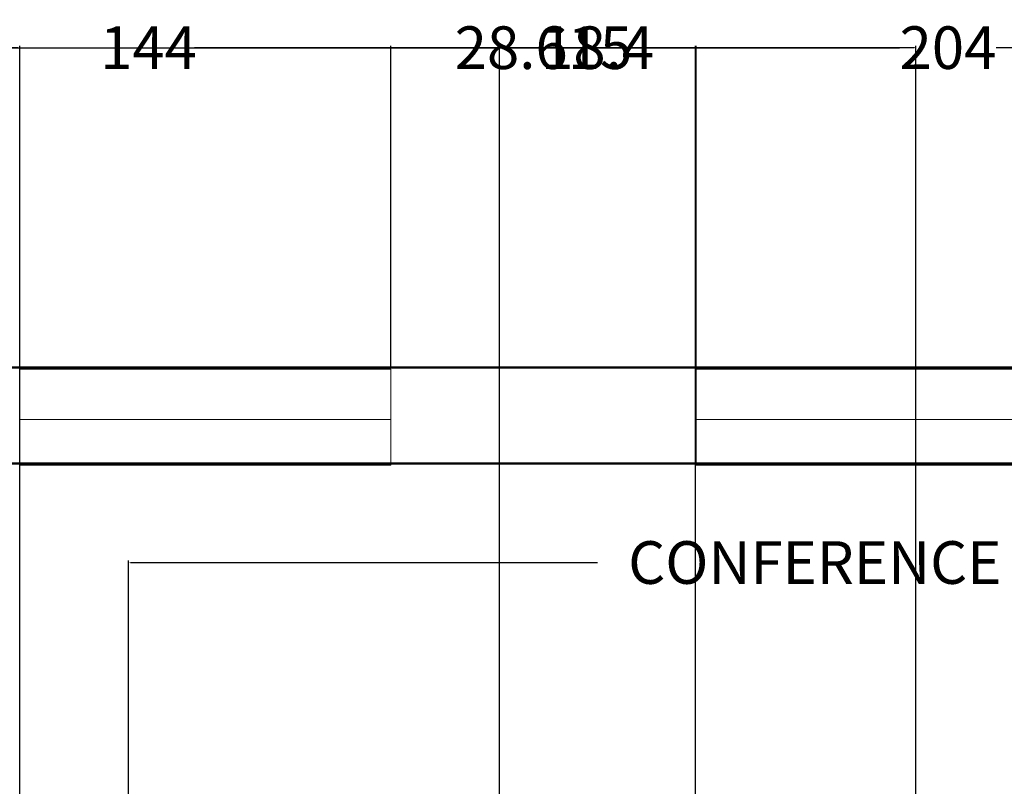
# Model space of a CAD drawing. Units: inches. Extents: x 1454 to 2136, y 626 to 1213.
# Tile 12 of 23: x 1561 to 1654, y 1141 to 1213. Entities that reach past the tile are written whole.
import ezdxf

# ---------------------------------------------------------------- set-up
doc = ezdxf.new("R2010")
doc.units = ezdxf.units.IN
doc.header["$MEASUREMENT"] = 0
for name, color, linetype, lineweight in [('A-ANNO-DIMS', 2, 'Continuous', 18), ('A-GLAZ', 4, 'Continuous', 18), ('A-WALL', 7, 'Continuous', 50)]:
    doc.layers.add(name, color=color, linetype=linetype, lineweight=lineweight)
doc.styles.get("Standard").update_dxf_attribs({"font": 'arial.ttf'})
doc.dimstyles.get("Standard").update_dxf_attribs({"dimtxt": 4, "dimasz": 0.18, "dimexe": 0.18, "dimexo": 0.0625, "dimgap": 0.09, "dimtad": 0, "dimtih": 1, "dimtoh": 1, "dimdec": 0, "dimrnd": 6, "dimzin": 0, "dimdsep": 46, "dimlunit": 3, "dimtxsty": 'Standard', "dimcen": 0.09, "dimadec": 0, "dimazin": 0, "dimtfac": 1, "dimtdec": 0, "dimtofl": 0, "dimtmove": 0, "dimatfit": 3, "dimfxl": 1, "dimtolj": 1, "dimtzin": 0, "dimarcsym": 0})

# ---------------------------------------------------------------- blocks, each defined once
blk = doc.blocks.new('WIN-34_84')
blk.add_line((34.84, 4.305), (0, 4.305))
blk.add_lwpolyline([(34.84, 0), (0, 0), (0, 9), (34.84, 9)], close=True)
blk = doc.blocks.new('*D23')
at = {"layer": 'A-ANNO-DIMS', "color": 0, "lineweight": -2, "transparency": 16777216}
for p, q in [((1571.674, 1139.532), (1571.674, 1162.157)), ((1571.854, 1161.977), (1615.675, 1161.977)), ((1721.545, 1161.977), (1677.724, 1161.977)), ((1721.725, 1139.532), (1721.725, 1162.157))]:
    blk.add_line(p, q, dxfattribs=at)
at = {"layer": 'A-ANNO-DIMS', "color": 0, "transparency": 16777216}
for points in [[(1571.854, 1162.007), (1571.854, 1161.947), (1571.674, 1161.977)], [(1721.545, 1162.007), (1721.545, 1161.947), (1721.725, 1161.977)]]:
    blk.add_solid(points, dxfattribs=at)
at = {"layer": 'Defpoints', "color": 0, "transparency": 16777216}
for p in [(1721.725, 1161.977), (1571.674, 1139.469), (1721.725, 1139.469)]:
    blk.add_point(p, dxfattribs=at)
at = {"layer": 'A-ANNO-DIMS', "color": 0, "transparency": 16777216, "insert": (1646.7, 1161.977), "char_height": 4, "attachment_point": 5}
blk.add_mtext('\\A1;CONFERENCE SET 150', dxfattribs=at)
blk = doc.blocks.new('*D29')
at = {"layer": 'A-ANNO-DIMS', "color": 0, "lineweight": -2, "transparency": 16777216}
for p, q in [((1546.556, 1171.345), (1546.556, 1210.464)), ((1546.736, 1210.284), (1644.022, 1210.284)), ((1750.376, 1210.284), (1653.091, 1210.284)), ((1750.556, 1171.345), (1750.556, 1210.464))]:
    blk.add_line(p, q, dxfattribs=at)
at = {"layer": 'A-ANNO-DIMS', "color": 0, "transparency": 16777216}
for points in [[(1546.736, 1210.314), (1546.736, 1210.254), (1546.556, 1210.284)], [(1750.376, 1210.314), (1750.376, 1210.254), (1750.556, 1210.284)]]:
    blk.add_solid(points, dxfattribs=at)
at = {"layer": 'Defpoints', "color": 0, "transparency": 16777216}
for p in [(1750.556, 1210.284), (1546.556, 1171.282), (1750.556, 1171.282)]:
    blk.add_point(p, dxfattribs=at)
at = {"layer": 'A-ANNO-DIMS', "color": 0, "transparency": 16777216, "insert": (1648.556, 1210.284), "char_height": 4, "attachment_point": 5}
blk.add_mtext('\\A1;204', dxfattribs=at)
blk = doc.blocks.new('*D40')
at = {"layer": 'A-ANNO-DIMS', "color": 0, "lineweight": -2, "transparency": 16777216}
for p, q in [((1501.556, 877.345), (1501.556, 1210.464)), ((1501.736, 1210.284), (1569.244, 1210.284)), ((1645.376, 1210.284), (1577.869, 1210.284)), ((1645.556, 877.345), (1645.556, 1210.464))]:
    blk.add_line(p, q, dxfattribs=at)
at = {"layer": 'A-ANNO-DIMS', "color": 0, "transparency": 16777216}
for points in [[(1501.736, 1210.314), (1501.736, 1210.254), (1501.556, 1210.284)], [(1645.376, 1210.314), (1645.376, 1210.254), (1645.556, 1210.284)]]:
    blk.add_solid(points, dxfattribs=at)
at = {"layer": 'Defpoints', "color": 0, "transparency": 16777216}
for p in [(1645.556, 1210.284), (1501.556, 877.282), (1645.556, 877.282)]:
    blk.add_point(p, dxfattribs=at)
at = {"layer": 'A-ANNO-DIMS', "color": 0, "transparency": 16777216, "insert": (1573.556, 1210.284), "char_height": 4, "attachment_point": 5}
blk.add_mtext('\\A1;144', dxfattribs=at)
blk = doc.blocks.new('*D50')
at = {"layer": 'A-ANNO-DIMS', "color": 0, "lineweight": -2, "transparency": 16777216}
for p, q in [((1596.305, 1180.166), (1596.305, 1210.464)), ((1596.485, 1210.284), (1602.17, 1210.284)), ((1624.74, 1210.284), (1619.054, 1210.284)), ((1624.92, 1180.166), (1624.92, 1210.464))]:
    blk.add_line(p, q, dxfattribs=at)
at = {"layer": 'A-ANNO-DIMS', "color": 0, "transparency": 16777216}
for points in [[(1596.485, 1210.314), (1596.485, 1210.254), (1596.305, 1210.284)], [(1624.74, 1210.314), (1624.74, 1210.254), (1624.92, 1210.284)]]:
    blk.add_solid(points, dxfattribs=at)
at = {"layer": 'Defpoints', "color": 0, "transparency": 16777216}
for p in [(1624.92, 1210.284), (1596.305, 1180.104), (1624.92, 1180.104)]:
    blk.add_point(p, dxfattribs=at)
at = {"layer": 'A-ANNO-DIMS', "color": 0, "transparency": 16777216, "insert": (1610.612, 1210.284), "char_height": 4, "attachment_point": 5}
blk.add_mtext('\\A1;28.615', dxfattribs=at)
blk = doc.blocks.new('*D55')
at = {"layer": 'A-ANNO-DIMS', "color": 0, "lineweight": -2, "transparency": 16777216}
for p, q in [((1537.556, 1018.345), (1537.556, 1210.464)), ((1537.736, 1210.284), (1542.647, 1210.284)), ((1561.304, 1210.284), (1556.393, 1210.284)), ((1561.484, 1018.345), (1561.484, 1210.464))]:
    blk.add_line(p, q, dxfattribs=at)
at = {"layer": 'A-ANNO-DIMS', "color": 0, "transparency": 16777216}
for points in [[(1537.736, 1210.314), (1537.736, 1210.254), (1537.556, 1210.284)], [(1561.304, 1210.314), (1561.304, 1210.254), (1561.484, 1210.284)]]:
    blk.add_solid(points, dxfattribs=at)
at = {"layer": 'Defpoints', "color": 0, "transparency": 16777216}
for p in [(1561.484, 1210.284), (1537.556, 1018.282), (1561.484, 1018.282)]:
    blk.add_point(p, dxfattribs=at)
at = {"layer": 'A-ANNO-DIMS', "color": 0, "transparency": 16777216, "insert": (1549.52, 1210.284), "char_height": 4, "attachment_point": 5}
blk.add_mtext('\\A1;23.93', dxfattribs=at)
blk = doc.blocks.new('*D67')
at = {"layer": 'A-ANNO-DIMS', "color": 0, "lineweight": -2, "transparency": 16777216}
for p, q in [((1606.484, 1018.345), (1606.484, 1210.464)), ((1606.664, 1210.284), (1610.595, 1210.284)), ((1624.703, 1210.284), (1620.773, 1210.284)), ((1624.883, 1018.329), (1624.883, 1210.464))]:
    blk.add_line(p, q, dxfattribs=at)
at = {"layer": 'A-ANNO-DIMS', "color": 0, "transparency": 16777216}
for points in [[(1606.664, 1210.314), (1606.664, 1210.254), (1606.484, 1210.284)], [(1624.703, 1210.314), (1624.703, 1210.254), (1624.883, 1210.284)]]:
    blk.add_solid(points, dxfattribs=at)
at = {"layer": 'Defpoints', "color": 0, "transparency": 16777216}
for p in [(1624.883, 1210.284), (1606.484, 1018.282), (1624.883, 1018.267)]:
    blk.add_point(p, dxfattribs=at)
at = {"layer": 'A-ANNO-DIMS', "color": 0, "transparency": 16777216, "insert": (1615.684, 1210.284), "char_height": 4, "attachment_point": 5}
blk.add_mtext('\\A1;18.4', dxfattribs=at)

msp = doc.modelspace()

# ---------------------------------------------------------------- linework, layer by layer
at = {"layer": 'A-WALL'}
for p, q in [((1759.5563, 1180.2825), (1537.5563, 1180.2825)), ((1750.5563, 1171.2825), (1546.5563, 1171.2825))]:
    msp.add_line(p, q, dxfattribs=at)

# ---------------------------------------------------------------- block references
at = {"layer": 'A-GLAZ'}
for p in [(1561.4646, 1171.1038), (1624.9195, 1171.1038)]:
    msp.add_blockref('WIN-34_84', p, dxfattribs=at)

# ---------------------------------------------------------------- dimensions: what is measured, and where the dimension line sits
at = {"layer": 'A-ANNO-DIMS'}
for base, p1, p2, override, picture, middle in [((1645.5563, 1210.2845), (1501.5563, 877.2825), (1645.5563, 877.2825), {"dimdec": 0, "dimlfac": 1, "dimrnd": 0, "dimzin": 0, "dimdsep": 46, "dimlunit": 2}, '*D40', (1573.5563, 1210.2845)), ((1561.4844, 1210.2845), (1537.5563, 1018.2825), (1561.4844, 1018.2825), {"dimdec": 2, "dimlfac": 1, "dimrnd": 0, "dimzin": 0, "dimdsep": 46, "dimlunit": 2}, '*D55', (1549.5203, 1210.2845)), ((1750.5563, 1210.2845), (1546.5563, 1171.2825), (1750.5563, 1171.2825), {"dimdec": 0, "dimlfac": 1, "dimrnd": 0, "dimzin": 0, "dimdsep": 46, "dimlunit": 2}, '*D29', (1648.5563, 1210.2845)), ((1624.9195, 1210.2845), (1596.3048, 1180.1038), (1624.9195, 1180.1038), {"dimdec": 3, "dimlfac": 1, "dimrnd": 0, "dimzin": 0, "dimdsep": 46, "dimlunit": 2}, '*D50', (1610.6122, 1210.2845)), ((1624.8835, 1210.2845), (1606.4844, 1018.2825), (1624.8835, 1018.2667), {"dimdec": 1, "dimlfac": 1, "dimrnd": 0, "dimzin": 0, "dimdsep": 46, "dimlunit": 2}, '*D67', (1615.6839, 1210.2845))]:
    dim = msp.add_linear_dim(base=base, p1=p1, p2=p2, dimstyle='Standard', override=override, dxfattribs=at)
    dim.commit()
    dim.dimension.update_dxf_attribs({"geometry": picture, "text_midpoint": middle})
dim = msp.add_linear_dim(base=(1721.7253, 1161.9768), p1=(1571.674, 1139.4691), p2=(1721.7253, 1139.4691), text='CONFERENCE SET <>', dimstyle='Standard', override={"dimdec": 0, "dimlfac": 1, "dimrnd": 0, "dimzin": 0, "dimdsep": 46, "dimlunit": 2}, dxfattribs=at)
dim.commit()
dim.dimension.update_dxf_attribs({"geometry": '*D23', "text_midpoint": (1646.6996, 1161.9768)})

doc.saveas('drawing.dxf')
